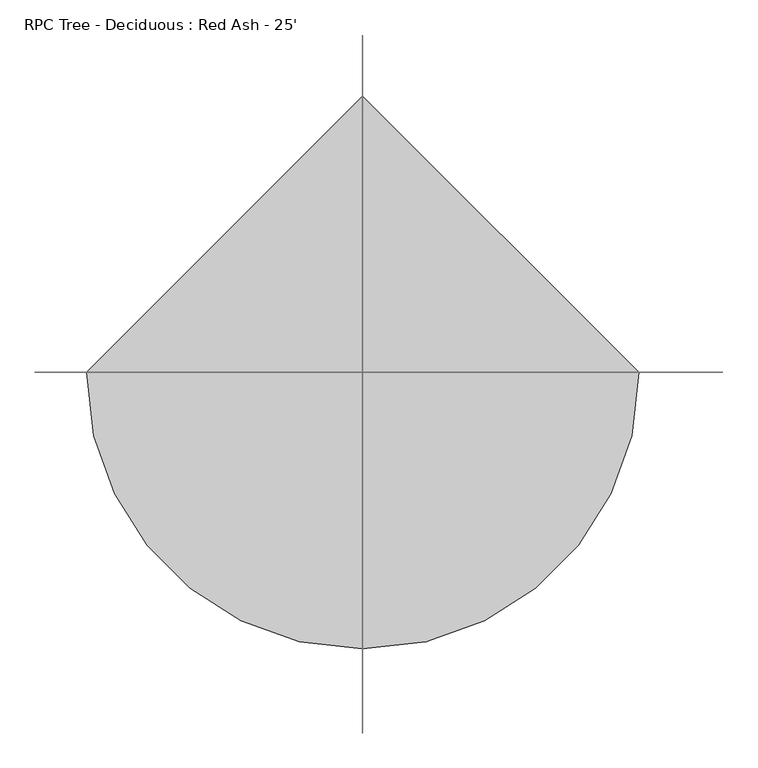
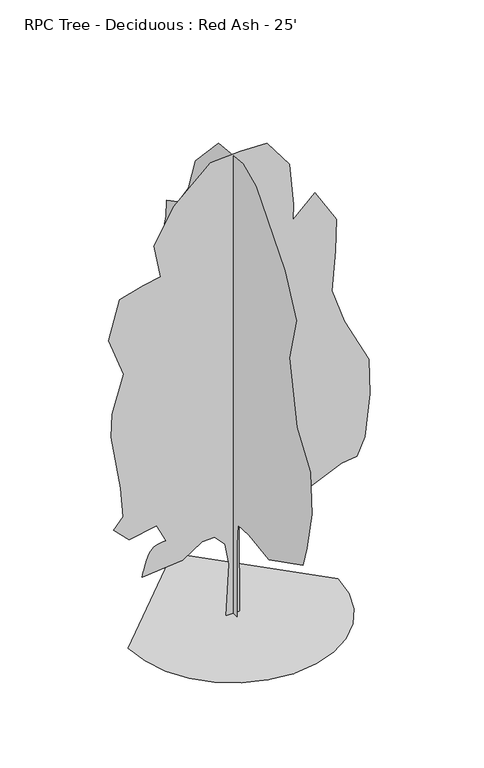
"""IFC4 building model written with IfcOpenShell, lengths in millimetres: geographic element geometry, RPC Tree - Deciduous : Red Ash - 25'."""

from ifc_helpers import new_model, si_unit, origin, place, context, project, spatial, triangles, source, transform, mapped, element, save


def rpc_tree_deciduous_red_ash_25_5dd3353f(model_context):
    return source(origin(), model_context, "Body", "Tessellation", [
        triangles([(-657.9809858, 0.0, 2.47e-05), (-640.5860447, -150.7657429, 2.47e-05), (-591.0457546, -289.2199553, 2.47e-05), (-513.3265523, -411.3957464, 2.47e-05), (-411.3957828, -513.3266613, 2.47e-05), (-289.2198827, -591.0456093, 2.47e-05), (-150.7656703, -640.5860447, 2.47e-05), (2.88e-05, -657.9809858, 2.47e-05), (150.765752, -640.5861174, 2.47e-05), (289.2199735, -591.0457183, 2.47e-05), (411.3957828, -513.3265523, 2.47e-05), (513.326734, -411.3957828, 2.47e-05), (591.045682, -289.2198645, 2.47e-05), (640.5860447, -150.7656339, 2.47e-05), (657.9809858, 5.75e-05, 2.47e-05), (-8.63e-05, 657.9809858, 2.47e-05), (-4.3e-06, -41.1385046, 0.0), (1e-05, -40.4986863, 477.8216337), (1.29e-05, -51.9527836, 615.1211746), (3e-07, -175.5301652, 623.2661716), (-2.31e-05, -390.5565024, 591.3227726), (-5.62e-05, -761.4770668, 779.4708086), (-5.65e-05, -804.4823633, 919.2380768), (-5.44e-05, -858.2390385, 1177.2697105), (-4.47e-05, -842.1121885, 1446.0528683), (-2.32e-05, -696.1527838, 1656.406889), (-2.2e-06, -610.9594374, 2064.2539421), (-1.4e-06, -686.2180704, 2354.5395664), (1.92e-05, -562.5780155, 2612.5713455), (6.28e-05, -250.7897429, 2983.4920189), (7.94e-05, -109.2802846, 3047.2776604), (0.0001065, 157.7606466, 3021.1216988), (0.0001248, 410.4167364, 2752.3386864), (0.000126, 485.6760962, 2526.5608978), (0.0001329, 598.5645181, 2365.2909451), (0.0001439, 722.2052633, 2300.7831093), (0.0001413, 727.58088, 2193.269759), (0.0001409, 759.8349432, 2069.6296314), (0.000131, 706.0782681, 1924.4868919), (0.0001319, 754.4592539, 1784.7196964), (0.0001312, 802.840167, 1591.1958984), (0.0001284, 792.0889338, 1537.4391506), (0.0001151, 700.7027241, 1408.4231884), (0.0001092, 694.9245884, 1231.0264584), (0.0001053, 689.9512728, 1118.1374914), (0.0001017, 695.3269621, 978.3704412), (9.65e-05, 700.7027241, 784.8467159), (8.69e-05, 625.443437, 725.7142788), (7.23e-05, 485.6762778, 725.7142788), (7.31e-05, 550.1842226, 526.8148642), (6.86e-05, 539.398035, 413.9538025), (6.07e-05, 441.2124221, 491.1345566), (3.95e-05, 251.7850674, 442.6830445), (3.92e-05, 220.684731, 542.8243884), (2.51e-05, 86.3651045, 541.6010256), (2.01e-05, 52.3204937, 491.3338177), (1.31e-05, 31.8197329, 327.3132697), (4.7e-06, 44.8664066, 5.1e-06), (-44.3483468, 1.9e-06, 1.78e-05), (-26.6845903, -3.86e-05, 333.4006525), (-51.7229194, -5.44e-05, 475.1774274), (-116.3151477, -6e-05, 546.1270575), (-193.4545798, -5.63e-05, 543.4785273), (-318.5071212, -4.12e-05, 462.3069194), (-571.163211, -2.76e-05, 440.8043438), (-567.6682571, -2.94e-05, 454.7058572), (-563.9382159, -3.13e-05, 469.0775454), (-559.7379999, -3.33e-05, 484.3894741), (-554.8325217, -3.55e-05, 501.1121452), (-548.9867303, -3.8e-05, 519.7150795), (-541.9654655, -4.08e-05, 540.6693601), (-533.5336764, -4.4e-05, 564.444435), (-522.9077625, -4.71e-05, 586.4957053), (-509.7428321, -4.96e-05, 602.6226643), (-494.4621878, -5.16e-05, 613.8126789), (-477.4888052, -5.32e-05, 621.053516), (-459.246096, -5.45e-05, 625.3319613), (-440.1569269, -5.56e-05, 627.6358177), (-420.6446732, -5.66e-05, 628.9523798), (-479.7768559, -6.81e-05, 747.2169634), (-651.798151, -5.67e-05, 714.9629728), (-748.5599047, -6.4e-05, 811.7250172), (-689.4276129, -7.5e-05, 881.6086149), (-705.5546082, -9.73e-05, 1075.1324129), (-764.6868273, -0.0001377, 1435.3014896), (-759.3923103, -0.0001557, 1584.466222), (-687.9670189, -0.0001875, 1825.330299), (-780.8138952, -0.0002139, 2080.3808647), (-710.9301521, -0.0002464, 2327.6614105), (-565.7874853, -0.0002579, 2370.6666344), (-455.3653009, -0.000265, 2390.1449512), (-495.9039602, -0.0002891, 2607.1958015), (-372.2636147, -0.0003208, 2827.5980461), (-141.1101186, -0.0003559, 3037.248912), (47.037872, -0.0003654, 3048.0), (213.6834868, -0.000372, 3042.6241653), (353.4506641, -0.0003557, 2854.4763474), (379.1488412, -0.000324, 2579.0071152), (375.4587685, -0.0003118, 2477.9879906), (514.7204352, -0.0003333, 2607.1958015), (649.1120504, -0.0003129, 2386.793557), (643.7363611, -0.0002878, 2178.6037937), (619.7830267, -0.000256, 1920.2608418), (697.4929636, -0.0002323, 1693.3332687), (852.7056553, -0.0002027, 1387.6792511), (857.6541904, -0.0001754, 1157.1237745), (826.5087805, -0.0001412, 881.6084696), (778.1278673, -0.0001257, 768.7195753), (681.3658957, -0.0001201, 757.9682693), (493.2178596, -0.0001017, 671.9576763), (326.5722176, -8.03e-05, 553.6931291), (102.9906158, -8.2e-05, 649.8275591), (37.220348, -7.07e-05, 579.0538994), (41.6620963, -1.8e-06, 1.41e-05)], [[15, 16, 1], [14, 15, 1], [14, 1, 2], [13, 14, 2], [13, 2, 3], [13, 3, 4], [12, 13, 4], [11, 12, 4], [11, 4, 5], [11, 5, 6], [11, 6, 7], [11, 7, 8], [11, 8, 9], [11, 9, 10], [50, 51, 52], [57, 58, 17], [57, 17, 18], [56, 57, 18], [56, 18, 19], [55, 56, 19], [49, 50, 52], [52, 53, 54], [49, 52, 54], [35, 36, 37], [46, 47, 48], [46, 48, 49], [21, 22, 23], [20, 21, 23], [20, 23, 24], [20, 24, 25], [20, 25, 26], [19, 20, 26], [19, 26, 27], [45, 46, 49], [31, 32, 33], [30, 31, 33], [29, 30, 33], [29, 33, 34], [28, 29, 34], [27, 28, 34], [19, 27, 34], [19, 34, 35], [19, 35, 37], [19, 37, 38], [19, 38, 39], [19, 39, 40], [19, 40, 41], [19, 41, 42], [19, 42, 43], [19, 43, 44], [19, 44, 45], [19, 45, 49], [19, 49, 54], [55, 19, 54], [64, 65, 66], [64, 66, 67], [64, 67, 68], [99, 100, 101], [64, 68, 69], [64, 69, 70], [64, 70, 71], [114, 59, 60], [113, 114, 60], [113, 60, 61], [113, 61, 62], [64, 71, 72], [64, 72, 73], [64, 73, 74], [64, 74, 75], [64, 75, 76], [64, 76, 77], [64, 77, 78], [64, 78, 79], [63, 64, 79], [81, 82, 83], [80, 81, 83], [99, 101, 102], [107, 108, 109], [110, 111, 112], [88, 89, 90], [87, 88, 90], [87, 90, 91], [80, 83, 84], [95, 96, 97], [95, 97, 98], [94, 95, 98], [93, 94, 98], [92, 93, 98], [91, 92, 98], [91, 98, 99], [87, 91, 99], [87, 99, 102], [87, 102, 103], [87, 103, 104], [86, 87, 104], [85, 86, 104], [84, 85, 104], [80, 84, 104], [80, 104, 105], [80, 105, 106], [80, 106, 107], [80, 107, 109], [80, 109, 110], [80, 110, 112], [79, 80, 112], [63, 79, 112], [62, 63, 112], [113, 62, 112]], closed=False),
    ])


if __name__ == "__main__":
    model = new_model("IFC4")
    model_context = context("Model", 3, world=origin())
    ifc_project = project(units=[si_unit("LENGTHUNIT", "METRE", prefix="MILLI")], contexts=[model_context])
    site = spatial("IfcSite", under=ifc_project)
    building = spatial("IfcBuilding", under=site)
    placement = place(None, origin())
    rpc_tree_deciduous_red_ash_25_shape = rpc_tree_deciduous_red_ash_25_5dd3353f(model_context)
    element("IfcGeographicElement", 1, ObjectType="RPC Tree - Deciduous : Red Ash - 25'", at=placement, inside=building, context=model_context, shape_type="MappedRepresentation", body=[
        mapped(rpc_tree_deciduous_red_ash_25_shape, transform((0.0, 0.0, 0.0), x_axis=(1.0, 0.0, 0.0), y_axis=(0.0, 1.0, 0.0), z_axis=(0.0, 0.0, 1.0))),
    ])
    save(model, "model.ifc")

# Revit data of these elements
# Type "RPC Tree - Deciduous : Red Ash - 25'"
#   built-in parameter 1005198 = "{2, 15},{22, RPC-8-G3GR-497X-PHW5-6},{1, 0},{1, 0},{2, 15},{1, 8},{5, Color},{1, 0},{1, 0},{3, 0.8},{3, 0.8},{3, 0.8},{1, 8},{7, BBoxMin},{1, 0},{1, 0},{1, 0},{1, 0},{1, 0},{1, 8},{7, BBoxMax},{1, 0},{1, 0},{1, 0},{1, 0},{1, 0},{2, 11},{9, RPCTypeId},{1, 0},{1, 0},{22, RPC-8-G3GR-497X-PHW5-6},{1, 6},{14, RPCPlantHeight},{1, 0},{1, 0},{2, 25},{2, 11},{7, keyword},{1, 0},{1, 0},{34, :RPCs:Trees [General]:Geometry:RPC},{2, 11},{8, category},{1, 0},{1, 0},{15, Trees [General]},{2, 11},{12, LocalizedUID},{1, 0},{1, 0},{7, Red Ash},{2, 14},{6, Height},{1, 0},{1, 0},{2, 25},{1, 2},{16, Cast Reflections},{1, 0},{1, 0},{1, 0},{1, 2},{6, Jitter},{1, 0},{1, 0},{1, 1},{1, 2},{9, Billboard},{1, 0},{1, 0},{1, 0},{1, 2},{12, Cast Shadows},{1, 0},{1, 0},{1, 1},{1, 2},{20, Apply Filter Effects},{1, 0},{1, 0},{1, 0},{2, 11},{28, Apply Filter Effects-Text-FC},{1, 0},{1, 0},{4, None},{21, assetlibrary_base.fbx},{1, 5},"
#   built-in parameter 1005195 = "RPC-8-G3GR-497X-PHW5-6"
#   Type Comments = "Red Maple"
#   Assembly Code = "G2050500"
#   Height = 10' - 0"
#   Default Elevation = 0
